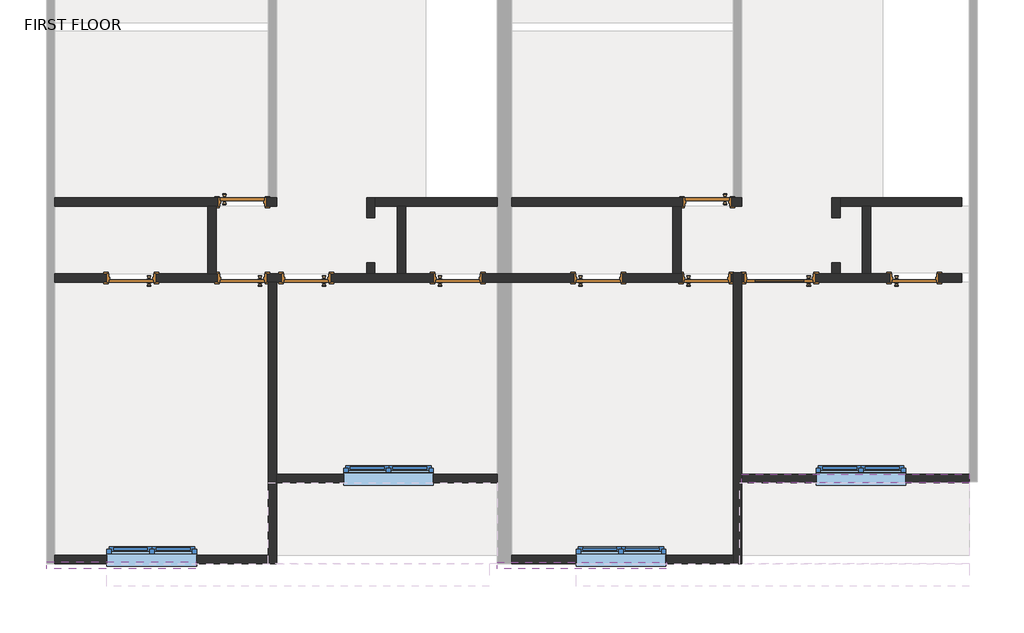
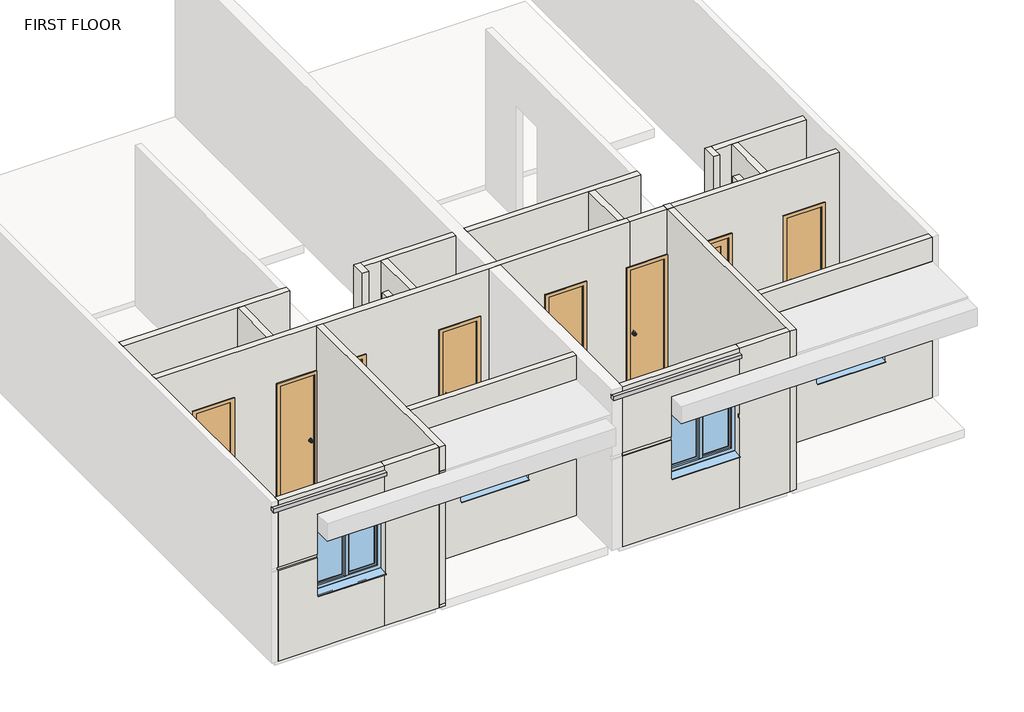
# One storey, part 1 of 2: 26 walls, 10 doors, 4 windows, 2 proxies.
"""IFC4 building model written with IfcOpenShell, lengths in millimetres."""

from ifc_helpers import new_model, si_unit, frame, origin, place, context, project, spatial, polyline, outline, extrude, faceted_brep, transform, mapped, element, save
from components import door_d4071c8b, door_c25f678d, door_03233f92, w2_0001_w2_2_f00e904a, w2_0001_w2_3_7b164e2c

model = new_model("IFC4")

# Units and contexts
model_context = context("Model", 3, world=origin())
ifc_project = project(units=[si_unit("LENGTHUNIT", "METRE", prefix="MILLI")], contexts=[model_context])

# Site, building, storey
site = spatial("IfcSite", under=ifc_project)
building = spatial("IfcBuilding", under=site)
storey = spatial("IfcBuildingStorey", under=building, Name="FIRST FLOOR", Elevation=3352.8)

# Proxies
placement = place(None, origin())
element("IfcBuildingElementProxy", 1, Name="Reveal 2", ObjectType="Reveal 2", at=placement, inside=storey, context=model_context, shape_type="SweptSolid", body=[
    extrude(outline(polyline([(-18263.2007021, -5496.2840801), (-18263.2007021, -5404.2090801), (-16237.550702, -5404.2090801), (-16237.550702, -5496.2840801), (-18263.2007021, -5496.2840801)])), frame((0.0, 0.0, 6248.4), z_axis=(0.0, 0.0, 1.0), x_axis=(1.0, 0.0, 0.0)), (0.0, 0.0, 1.0), 67.7333333),
])
element("IfcBuildingElementProxy", 2, Name="Reveal 2", ObjectType="Reveal 2", at=placement, inside=storey, context=model_context, shape_type="SweptSolid", body=[
    extrude(outline(polyline([(-9849.450702, -5405.2582515), (-9849.450702, -5497.3332515), (-12149.0934009, -5497.3332515), (-12149.0934009, -5405.2582515), (-9849.450702, -5405.2582515)])), frame((0.0, 0.0, 6248.4), z_axis=(0.0, 0.0, 1.0), x_axis=(1.0, 0.0, 0.0)), (0.0, 0.0, 1.0), 67.7333333),
])

# Doors
door_shape = door_d4071c8b(model_context)
element("IfcDoor", 3, ObjectType="Door-Interior-Single-2_Panel-Wood : 36\" x 84\"", at=placement, inside=storey, context=model_context, shape_type="MappedRepresentation", body=[
    mapped(door_shape, transform((-8312.7507021, -1552.9340801, 3352.8), x_axis=(-1.0, 0.0, 0.0), y_axis=(0.0, -1.0, 0.0), z_axis=(0.0, 0.0, 1.0))),
])
door_2_shape = door_c25f678d(model_context)
element("IfcDoor", 4, ObjectType="Door-Interior-Single-Flush_Panel-Wood : 24\" x 84\"", at=placement, inside=storey, context=model_context, shape_type="MappedRepresentation", body=[
    mapped(door_2_shape, transform((-17112.9480934, -1552.9340801, 3352.8), x_axis=(-1.0, 0.0, 0.0), y_axis=(0.0, -1.0, 0.0), z_axis=(0.0, 0.0, 1.0))),
])
element("IfcDoor", 5, ObjectType="Door-Interior-Single-Flush_Panel-Wood : 24\" x 84\"", at=placement, inside=storey, context=model_context, shape_type="MappedRepresentation", body=[
    mapped(door_2_shape, transform((-15607.9980934, -1552.9340801, 3352.8), x_axis=(-1.0, 0.0, 0.0), y_axis=(0.0, -1.0, 0.0), z_axis=(0.0, 0.0, 1.0))),
])
element("IfcDoor", 6, ObjectType="Door-Interior-Single-Flush_Panel-Wood : 24\" x 84\"", at=placement, inside=storey, context=model_context, shape_type="MappedRepresentation", body=[
    mapped(door_2_shape, transform((-14738.950702, -1552.9340801, 3352.8), x_axis=(-1.0, 0.0, 0.0), y_axis=(0.0, -1.0, 0.0), z_axis=(0.0, 0.0, 1.0))),
])
element("IfcDoor", 7, ObjectType="Door-Interior-Single-Flush_Panel-Wood : 24\" x 84\"", at=placement, inside=storey, context=model_context, shape_type="MappedRepresentation", body=[
    mapped(door_2_shape, transform((-15607.9980934, -517.8840801, 3352.8), x_axis=(1.0, 0.0, 0.0), y_axis=(0.0, 1.0, 0.0), z_axis=(0.0, 0.0, 1.0))),
])
door_3_shape = door_03233f92(model_context)
element("IfcDoor", 8, ObjectType="Door-Interior-Single-Flush_Panel-Wood : 24\" x 84\"", at=placement, inside=storey, context=model_context, shape_type="MappedRepresentation", body=[
    mapped(door_3_shape, transform((-9296.0980934, -517.8840801, 3352.8), x_axis=(-1.0, 0.0, 0.0), y_axis=(0.0, -1.0, 0.0), z_axis=(0.0, 0.0, 1.0))),
])
element("IfcDoor", 9, ObjectType="Door-Interior-Single-Flush_Panel-Wood : 24\" x 84\"", at=placement, inside=storey, context=model_context, shape_type="MappedRepresentation", body=[
    mapped(door_3_shape, transform((-9307.8954847, -1552.9340801, 3352.8), x_axis=(1.0, 0.0, 0.0), y_axis=(0.0, 1.0, 0.0), z_axis=(0.0, 0.0, 1.0))),
])
element("IfcDoor", 10, ObjectType="Door-Interior-Single-Flush_Panel-Wood : 24\" x 84\"", at=placement, inside=storey, context=model_context, shape_type="MappedRepresentation", body=[
    mapped(door_3_shape, transform((-10774.7454848, -1552.9340801, 3352.8), x_axis=(1.0, 0.0, 0.0), y_axis=(0.0, 1.0, 0.0), z_axis=(0.0, 0.0, 1.0))),
])
element("IfcDoor", 11, ObjectType="Door-Interior-Single-Flush_Panel-Wood : 24\" x 84\"", at=placement, inside=storey, context=model_context, shape_type="MappedRepresentation", body=[
    mapped(door_3_shape, transform((-6487.1257021, -1552.9340801, 3352.8), x_axis=(1.0, 0.0, 0.0), y_axis=(0.0, 1.0, 0.0), z_axis=(0.0, 0.0, 1.0))),
])
element("IfcDoor", 12, ObjectType="Door-Interior-Single-Flush_Panel-Wood : 24\" x 84\"", at=placement, inside=storey, context=model_context, shape_type="MappedRepresentation", body=[
    mapped(door_3_shape, transform((-12681.5507021, -1552.9340801, 3352.8), x_axis=(1.0, 0.0, 0.0), y_axis=(0.0, 1.0, 0.0), z_axis=(0.0, 0.0, 1.0))),
])

# Walls
element("IfcWall", 13, at=placement, inside=storey, context=model_context, shape_type="Brep", body=[
    faceted_brep([(-15139.0007021, -578.2090801, 6400.8), (-15962.6954847, -578.2090801, 6400.8), (-16076.9954847, -578.2090801, 6400.8), (-18148.9007021, -578.2090801, 6400.8), (-18148.9007021, -578.2090801, 3352.8), (-16076.9954847, -578.2090801, 3352.8), (-15962.6954847, -578.2090801, 3352.8), (-15938.1980934, -578.2090801, 3352.8), (-15938.1980934, -578.2090801, 5511.8), (-15277.7980934, -578.2090801, 5511.8), (-15277.7980934, -578.2090801, 3352.8), (-15139.0007021, -578.2090801, 3352.8), (-18148.9007021, -463.9090801, 6400.8), (-15253.3007021, -463.9090801, 6400.8), (-15139.0007021, -463.9090801, 6400.8), (-15139.0007021, -463.9090801, 3352.8), (-15253.3007021, -463.9090801, 3352.8), (-15277.7980934, -463.9090801, 3352.8), (-15277.7980934, -463.9090801, 5511.8), (-15938.1980934, -463.9090801, 5511.8), (-15938.1980934, -463.9090801, 3352.8), (-18148.9007021, -463.9090801, 3352.8)], [[[0, 1, 2, 3, 4, 5, 6, 7, 8, 9, 10, 11]], [[12, 13, 14, 15, 16, 17, 18, 19, 20, 21]], [[4, 21, 20, 7, 6, 5]], [[15, 11, 10, 17, 16]], [[3, 2, 1, 0, 14, 13, 12]], [[4, 3, 12, 21]], [[0, 11, 15, 14]], [[9, 18, 17, 10]], [[18, 9, 8, 19]], [[19, 8, 7, 20]]]),
])
element("IfcWall", 14, at=placement, inside=storey, context=model_context, shape_type="Brep", body=[
    faceted_brep([(-9612.6954847, -1606.9090801, 6400.8), (-11945.8934009, -1606.9090801, 6400.8), (-12149.0934009, -1606.9090801, 6400.8), (-15139.000702, -1606.9090801, 6400.8), (-15253.300702, -1606.9090801, 6400.8), (-18148.9007021, -1606.9090801, 6400.8), (-18148.9007021, -1606.9090801, 3352.8), (-17443.1480934, -1606.9090801, 3352.8), (-17443.1480934, -1606.9090801, 5511.8), (-16782.7480934, -1606.9090801, 5511.8), (-16782.7480934, -1606.9090801, 3352.8), (-15938.1980934, -1606.9090801, 3352.8), (-15938.1980934, -1606.9090801, 5511.8), (-15277.7980934, -1606.9090801, 5511.8), (-15277.7980934, -1606.9090801, 3352.8), (-15253.300702, -1606.9090801, 3352.8), (-15139.000702, -1606.9090801, 3352.8), (-15069.150702, -1606.9090801, 3352.8), (-15069.150702, -1606.9090801, 5511.8), (-14408.750702, -1606.9090801, 5511.8), (-14408.750702, -1606.9090801, 3352.8), (-13011.7507021, -1606.9090801, 3352.8), (-13011.7507021, -1606.9090801, 5511.8), (-12351.3507021, -1606.9090801, 5511.8), (-12351.3507021, -1606.9090801, 3352.8), (-12149.0934009, -1606.9090801, 3352.8), (-11945.8934009, -1606.9090801, 3352.8), (-11104.9454848, -1606.9090801, 3352.8), (-11104.9454848, -1606.9090801, 5511.8), (-10444.5454848, -1606.9090801, 5511.8), (-10444.5454848, -1606.9090801, 3352.8), (-9638.0954847, -1606.9090801, 3352.8), (-9638.0954847, -1606.9090801, 5511.8), (-9612.6954847, -1606.9090801, 5511.8), (-18148.9007021, -1492.6090801, 6400.8), (-16076.9954847, -1492.6090801, 6400.8), (-15962.6954847, -1492.6090801, 6400.8), (-13919.8007021, -1492.6090801, 6400.8), (-13805.5007021, -1492.6090801, 6400.8), (-13500.7007021, -1492.6090801, 6400.8), (-13386.4007021, -1492.6090801, 6400.8), (-12149.0934009, -1492.6090801, 6400.8), (-11945.8934009, -1492.6090801, 6400.8), (-9765.0954848, -1492.6090801, 6400.8), (-9650.7954848, -1492.6090801, 6400.8), (-9612.6954847, -1492.6090801, 6400.8), (-9612.6954847, -1492.6090801, 5511.8), (-9638.0954847, -1492.6090801, 5511.8), (-9638.0954847, -1492.6090801, 3352.8), (-9650.7954848, -1492.6090801, 3352.8), (-9765.0954848, -1492.6090801, 3352.8), (-10444.5454848, -1492.6090801, 3352.8), (-10444.5454848, -1492.6090801, 5511.8), (-11104.9454848, -1492.6090801, 5511.8), (-11104.9454848, -1492.6090801, 3352.8), (-11945.8934009, -1492.6090801, 3352.8), (-12149.0934009, -1492.6090801, 3352.8), (-12351.3507021, -1492.6090801, 3352.8), (-12351.3507021, -1492.6090801, 5511.8), (-13011.7507021, -1492.6090801, 5511.8), (-13011.7507021, -1492.6090801, 3352.8), (-13386.4007021, -1492.6090801, 3352.8), (-13500.7007021, -1492.6090801, 3352.8), (-13805.5007021, -1492.6090801, 3352.8), (-13919.8007021, -1492.6090801, 3352.8), (-14408.750702, -1492.6090801, 3352.8), (-14408.750702, -1492.6090801, 5511.8), (-15069.150702, -1492.6090801, 5511.8), (-15069.150702, -1492.6090801, 3352.8), (-15277.7980934, -1492.6090801, 3352.8), (-15277.7980934, -1492.6090801, 5511.8), (-15938.1980934, -1492.6090801, 5511.8), (-15938.1980934, -1492.6090801, 3352.8), (-15962.6954847, -1492.6090801, 3352.8), (-16076.9954847, -1492.6090801, 3352.8), (-16782.7480934, -1492.6090801, 3352.8), (-16782.7480934, -1492.6090801, 5511.8), (-17443.1480934, -1492.6090801, 5511.8), (-17443.1480934, -1492.6090801, 3352.8), (-18148.9007021, -1492.6090801, 3352.8)], [[[0, 1, 2, 3, 4, 5, 6, 7, 8, 9, 10, 11, 12, 13, 14, 15, 16, 17, 18, 19, 20, 21, 22, 23, 24, 25, 26, 27, 28, 29, 30, 31, 32, 33]], [[34, 35, 36, 37, 38, 39, 40, 41, 42, 43, 44, 45, 46, 47, 48, 49, 50, 51, 52, 53, 54, 55, 56, 57, 58, 59, 60, 61, 62, 63, 64, 65, 66, 67, 68, 69, 70, 71, 72, 73, 74, 75, 76, 77, 78, 79]], [[6, 79, 78, 7]], [[10, 75, 74, 73, 72, 11]], [[14, 69, 68, 17, 16, 15]], [[20, 65, 64, 63, 62, 61, 60, 21]], [[48, 31, 30, 51, 50, 49]], [[54, 27, 26, 25, 24, 57, 56, 55]], [[45, 0, 33, 46]], [[5, 4, 3, 2, 1, 0, 45, 44, 43, 42, 41, 40, 39, 38, 37, 36, 35, 34]], [[6, 5, 34, 79]], [[77, 8, 7, 78]], [[8, 77, 76, 9]], [[9, 76, 75, 10]], [[71, 12, 11, 72]], [[12, 71, 70, 13]], [[13, 70, 69, 14]], [[67, 18, 17, 68]], [[18, 67, 66, 19]], [[19, 66, 65, 20]], [[32, 47, 46, 33]], [[47, 32, 31, 48]], [[29, 52, 51, 30]], [[52, 29, 28, 53]], [[53, 28, 27, 54]], [[23, 58, 57, 24]], [[58, 23, 22, 59]], [[59, 22, 21, 60]]]),
])
element("IfcWall", 15, at=placement, inside=storey, context=model_context, shape_type="SweptSolid", body=[
    extrude(outline(polyline([(-16076.9954847, -1492.6090801), (-16076.9954847, -578.2090801), (-15962.6954847, -578.2090801), (-15962.6954847, -1492.6090801), (-16076.9954847, -1492.6090801)])), frame((0.0, 0.0, 3352.8), z_axis=(0.0, 0.0, 1.0), x_axis=(1.0, 0.0, 0.0)), (0.0, 0.0, 1.0), 3048.0),
])
element("IfcWall", 16, at=placement, inside=storey, context=model_context, shape_type="Brep", body=[
    faceted_brep([(-15139.000702, -5429.6090801, 3352.8), (-15139.000702, -4329.734083, 3352.8), (-15139.000702, -4215.434083, 3352.8), (-15139.000702, -1606.9090801, 3352.8), (-15139.000702, -1606.9090801, 3403.6), (-15139.000702, -5429.6090801, 3403.6), (-15253.300702, -5429.6090801, 3352.8), (-15253.300702, -5429.6090801, 3403.6), (-15253.300702, -1606.9090801, 3403.6), (-15253.300702, -1606.9090801, 3352.8), (-15253.300702, -5315.3090801, 3352.8)], [[[0, 1, 2, 3, 4, 5]], [[6, 7, 8, 9, 10]], [[3, 2, 1, 0, 6, 10, 9]], [[5, 4, 8, 7]], [[4, 3, 9, 8]], [[0, 5, 7, 6]]]),
])
element("IfcWall", 17, at=placement, inside=storey, context=model_context, shape_type="Brep", body=[
    faceted_brep([(-8827.100702, -5430.6582515, 3352.8), (-8827.100702, -4329.7340831, 3352.8), (-8827.100702, -4215.4340831, 3352.8), (-8827.100702, -1479.9090801, 3352.8), (-8827.100702, -1479.9090801, 6400.8), (-8827.100702, -4215.4340831, 6400.8), (-8827.100702, -4329.7340831, 6400.8), (-8827.100702, -5430.6582515, 6400.8), (-8941.400702, -5430.6582515, 3352.8), (-8941.400702, -5430.6582515, 6400.8), (-8941.400702, -5316.3582515, 6400.8), (-8941.400702, -1479.9090801, 6400.8), (-8941.400702, -1479.9090801, 3352.8), (-8941.400702, -5316.3582515, 3352.8)], [[[0, 1, 2, 3, 4, 5, 6, 7]], [[8, 9, 10, 11, 12, 13]], [[3, 2, 1, 0, 8, 13, 12]], [[4, 3, 12, 11]], [[7, 6, 5, 4, 11, 10, 9]], [[0, 7, 9, 8]]]),
])
element("IfcWall", 18, at=placement, inside=storey, context=model_context, shape_type="Brep", body=[
    faceted_brep([(-8827.1007021, -578.2090801, 6400.8), (-9650.7954848, -578.2090801, 6400.8), (-9765.0954848, -578.2090801, 6400.8), (-11945.8934009, -578.2090801, 6400.8), (-11945.8934009, -578.2090801, 3352.8), (-9765.0954848, -578.2090801, 3352.8), (-9650.7954848, -578.2090801, 3352.8), (-9626.2980934, -578.2090801, 3352.8), (-9626.2980934, -578.2090801, 5511.8), (-8965.8980934, -578.2090801, 5511.8), (-8965.8980934, -578.2090801, 3352.8), (-8827.1007021, -578.2090801, 3352.8), (-11945.8934009, -463.9090801, 6400.8), (-8941.4007021, -463.9090801, 6400.8), (-8827.1007021, -463.9090801, 6400.8), (-8827.1007021, -463.9090801, 3352.8), (-8941.4007021, -463.9090801, 3352.8), (-8965.8980934, -463.9090801, 3352.8), (-8965.8980934, -463.9090801, 5511.8), (-9626.2980934, -463.9090801, 5511.8), (-9626.2980934, -463.9090801, 3352.8), (-11945.8934009, -463.9090801, 3352.8)], [[[0, 1, 2, 3, 4, 5, 6, 7, 8, 9, 10, 11]], [[12, 13, 14, 15, 16, 17, 18, 19, 20, 21]], [[4, 21, 20, 7, 6, 5]], [[15, 11, 10, 17, 16]], [[3, 2, 1, 0, 14, 13, 12]], [[4, 3, 12, 21]], [[0, 11, 15, 14]], [[19, 8, 7, 20]], [[8, 19, 18, 9]], [[9, 18, 17, 10]]]),
])
element("IfcWall", 19, at=placement, inside=storey, context=model_context, shape_type="SweptSolid", body=[
    extrude(outline(polyline([(-9650.7954848, -578.2090801), (-9650.7954848, -1492.6090801), (-9765.0954848, -1492.6090801), (-9765.0954848, -578.2090801), (-9650.7954848, -578.2090801)])), frame((0.0, 0.0, 3352.8), z_axis=(0.0, 0.0, 1.0), x_axis=(1.0, 0.0, 0.0)), (0.0, 0.0, 1.0), 3048.0),
])
element("IfcWall", 20, at=placement, inside=storey, context=model_context, shape_type="Brep", body=[
    faceted_brep([(-9612.6954847, -1492.6090801, 6400.8), (-7607.9007021, -1492.6090801, 6400.8), (-7493.6007021, -1492.6090801, 6400.8), (-7188.8007021, -1492.6090801, 6400.8), (-7074.5007021, -1492.6090801, 6400.8), (-5842.6007021, -1492.6090801, 6400.8), (-5842.6007021, -1492.6090801, 3352.8), (-6156.9257021, -1492.6090801, 3352.8), (-6156.9257021, -1492.6090801, 5511.8), (-6817.3257021, -1492.6090801, 5511.8), (-6817.3257021, -1492.6090801, 3352.8), (-7074.5007021, -1492.6090801, 3352.8), (-7188.8007021, -1492.6090801, 3352.8), (-7493.6007021, -1492.6090801, 3352.8), (-7607.9007021, -1492.6090801, 3352.8), (-7830.1507021, -1492.6090801, 3352.8), (-7830.1507021, -1492.6090801, 5511.8), (-8795.3507021, -1492.6090801, 5511.8), (-8795.3507021, -1492.6090801, 3352.8), (-8977.6954847, -1492.6090801, 3352.8), (-8977.6954847, -1492.6090801, 5511.8), (-9612.6954847, -1492.6090801, 5511.8), (-5842.6007021, -1606.9090801, 6400.8), (-9612.6954847, -1606.9090801, 6400.8), (-9612.6954847, -1606.9090801, 5511.8), (-8977.6954847, -1606.9090801, 5511.8), (-8977.6954847, -1606.9090801, 3352.8), (-8795.3507021, -1606.9090801, 3352.8), (-8795.3507021, -1606.9090801, 5511.8), (-7830.1507021, -1606.9090801, 5511.8), (-7830.1507021, -1606.9090801, 3352.8), (-6817.3257021, -1606.9090801, 3352.8), (-6817.3257021, -1606.9090801, 5511.8), (-6156.9257021, -1606.9090801, 5511.8), (-6156.9257021, -1606.9090801, 3352.8), (-5842.6007021, -1606.9090801, 3352.8)], [[[0, 1, 2, 3, 4, 5, 6, 7, 8, 9, 10, 11, 12, 13, 14, 15, 16, 17, 18, 19, 20, 21]], [[22, 23, 24, 25, 26, 27, 28, 29, 30, 31, 32, 33, 34, 35]], [[6, 35, 34, 7]], [[26, 19, 18, 27]], [[10, 31, 30, 15, 14, 13, 12, 11]], [[23, 0, 21, 24]], [[5, 4, 3, 2, 1, 0, 23, 22]], [[6, 5, 22, 35]], [[25, 20, 19, 26]], [[20, 25, 24, 21]], [[33, 8, 7, 34]], [[8, 33, 32, 9]], [[9, 32, 31, 10]], [[17, 28, 27, 18]], [[28, 17, 16, 29]], [[29, 16, 15, 30]]]),
])
element("IfcWall", 21, at=placement, inside=storey, context=model_context, shape_type="Brep", body=[
    faceted_brep([(-7493.6007021, -730.6090801, 3352.8), (-7493.6007021, -578.2090801, 3352.8), (-7493.6007021, -463.9090801, 3352.8), (-7493.6007021, -463.9090801, 6400.8), (-7493.6007021, -578.2090801, 6400.8), (-7493.6007021, -730.6090801, 6400.8), (-7607.9007021, -730.6090801, 3352.8), (-7607.9007021, -730.6090801, 6400.8), (-7607.9007021, -463.9090801, 6400.8), (-7607.9007021, -463.9090801, 3352.8)], [[[0, 1, 2, 3, 4, 5]], [[6, 7, 8, 9]], [[2, 1, 0, 6, 9]], [[5, 4, 3, 8, 7]], [[0, 5, 7, 6]], [[3, 2, 9, 8]]]),
])
element("IfcWall", 22, at=placement, inside=storey, context=model_context, shape_type="Brep", body=[
    faceted_brep([(-7493.6007021, -578.2090801, 3352.8), (-7188.8007021, -578.2090801, 3352.8), (-7074.5007021, -578.2090801, 3352.8), (-5842.6007021, -578.2090801, 3352.8), (-5842.6007021, -578.2090801, 6400.8), (-7074.5007021, -578.2090801, 6400.8), (-7188.8007021, -578.2090801, 6400.8), (-7493.6007021, -578.2090801, 6400.8), (-7493.6007021, -463.9090801, 3352.8), (-7493.6007021, -463.9090801, 6400.8), (-5842.6007021, -463.9090801, 6400.8), (-5842.6007021, -463.9090801, 3352.8)], [[[0, 1, 2, 3, 4, 5, 6, 7]], [[8, 9, 10, 11]], [[3, 2, 1, 0, 8, 11]], [[4, 3, 11, 10]], [[7, 6, 5, 4, 10, 9]], [[0, 7, 9, 8]]]),
])
element("IfcWall", 23, at=placement, inside=storey, context=model_context, shape_type="SweptSolid", body=[
    extrude(outline(polyline([(-7493.6007021, -1340.2090801), (-7493.6007021, -1492.6090801), (-7607.9007021, -1492.6090801), (-7607.9007021, -1340.2090801), (-7493.6007021, -1340.2090801)])), frame((0.0, 0.0, 3352.8), z_axis=(0.0, 0.0, 1.0), x_axis=(1.0, 0.0, 0.0)), (0.0, 0.0, 1.0), 3048.0),
])
element("IfcWall", 24, at=placement, inside=storey, context=model_context, shape_type="SweptSolid", body=[
    extrude(outline(polyline([(-7074.5007021, -578.2090801), (-7074.5007021, -1492.6090801), (-7188.8007021, -1492.6090801), (-7188.8007021, -578.2090801), (-7074.5007021, -578.2090801)])), frame((0.0, 0.0, 3352.8), z_axis=(0.0, 0.0, 1.0), x_axis=(1.0, 0.0, 0.0)), (0.0, 0.0, 1.0), 3048.0),
])
element("IfcWall", 25, at=placement, inside=storey, context=model_context, shape_type="SweptSolid", body=[
    extrude(outline(polyline([(-13386.4007021, -578.2090801), (-13386.4007021, -1492.6090801), (-13500.7007021, -1492.6090801), (-13500.7007021, -578.2090801), (-13386.4007021, -578.2090801)])), frame((0.0, 0.0, 3352.8), z_axis=(0.0, 0.0, 1.0), x_axis=(1.0, 0.0, 0.0)), (0.0, 0.0, 1.0), 3048.0),
])
element("IfcWall", 26, at=placement, inside=storey, context=model_context, shape_type="Brep", body=[
    faceted_brep([(-13805.5007021, -730.6090801, 3352.8), (-13805.5007021, -578.2090801, 3352.8), (-13805.5007021, -463.9090801, 3352.8), (-13805.5007021, -463.9090801, 6400.8), (-13805.5007021, -578.2090801, 6400.8), (-13805.5007021, -730.6090801, 6400.8), (-13919.8007021, -730.6090801, 3352.8), (-13919.8007021, -730.6090801, 6400.8), (-13919.8007021, -463.9090801, 6400.8), (-13919.8007021, -463.9090801, 3352.8)], [[[0, 1, 2, 3, 4, 5]], [[6, 7, 8, 9]], [[2, 1, 0, 6, 9]], [[5, 4, 3, 8, 7]], [[0, 5, 7, 6]], [[3, 2, 9, 8]]]),
])
element("IfcWall", 27, at=placement, inside=storey, context=model_context, shape_type="Brep", body=[
    faceted_brep([(-13805.5007021, -578.2090801, 3352.8), (-13500.7007021, -578.2090801, 3352.8), (-13386.4007021, -578.2090801, 3352.8), (-12149.0934009, -578.2090801, 3352.8), (-12149.0934009, -578.2090801, 6400.8), (-13386.4007021, -578.2090801, 6400.8), (-13500.7007021, -578.2090801, 6400.8), (-13805.5007021, -578.2090801, 6400.8), (-13805.5007021, -463.9090801, 3352.8), (-13805.5007021, -463.9090801, 6400.8), (-12149.0934009, -463.9090801, 6400.8), (-12149.0934009, -463.9090801, 3352.8)], [[[0, 1, 2, 3, 4, 5, 6, 7]], [[8, 9, 10, 11]], [[3, 2, 1, 0, 8, 11]], [[7, 6, 5, 4, 10, 9]], [[0, 7, 9, 8]], [[4, 3, 11, 10]]]),
])
element("IfcWall", 28, at=placement, inside=storey, context=model_context, shape_type="SweptSolid", body=[
    extrude(outline(polyline([(-13805.5007021, -1340.2090801), (-13805.5007021, -1492.6090801), (-13919.8007021, -1492.6090801), (-13919.8007021, -1340.2090801), (-13805.5007021, -1340.2090801)])), frame((0.0, 0.0, 3352.8), z_axis=(0.0, 0.0, 1.0), x_axis=(1.0, 0.0, 0.0)), (0.0, 0.0, 1.0), 3048.0),
])
element("IfcWall", 29, at=placement, inside=storey, context=model_context, shape_type="SweptSolid", body=[
    extrude(outline(polyline([(3352.8, -15139.000702), (3352.8, -12149.0934009), (6400.8, -12149.0934009), (6400.8, -15139.000702), (3352.8, -15139.000702)]), holes=[polyline([(4352.8, -13012.2220515), (4352.8, -14231.4220515), (5612.8, -14231.4220515), (5612.8, -13012.2220515), (4352.8, -13012.2220515)])]), frame((0.0, -4329.734083, 0.0), z_axis=(0.0, 1.0, 0.0), x_axis=(0.0, 0.0, 1.0)), (0.0, 0.0, 1.0), 114.3),
])
element("IfcWall", 30, at=placement, inside=storey, context=model_context, shape_type="Brep", body=[
    faceted_brep([(-18148.9007021, -5429.6090801, 3352.8), (-16237.550702, -5429.6090801, 3352.8), (-16237.550702, -5429.6090801, 4352.8), (-17444.0507021, -5429.6090801, 4352.8), (-17444.0507021, -5429.6090801, 5072.38), (-18148.9007021, -5429.6090801, 5072.38), (-16237.550702, -5429.6090801, 6400.8), (-18148.9007021, -5429.6090801, 6400.8), (-18148.9007021, -5429.6090801, 6316.1333333), (-16237.550702, -5429.6090801, 6316.1333333), (-17444.0507021, -5429.6090801, 5572.0), (-16237.550702, -5429.6090801, 5572.0), (-16237.550702, -5429.6090801, 6248.4), (-18148.9007021, -5429.6090801, 6248.4), (-18148.9007021, -5429.6090801, 5140.1133333), (-17444.0507021, -5429.6090801, 5140.1133333), (-16237.550702, -5315.3090801, 3352.8), (-18148.9007021, -5315.3090801, 3352.8), (-18148.9007021, -5315.3090801, 6400.8), (-16237.550702, -5315.3090801, 6400.8), (-16237.550702, -5315.3090801, 5572.0), (-17444.0507021, -5315.3090801, 5572.0), (-17444.0507021, -5315.3090801, 4352.8), (-16237.550702, -5315.3090801, 4352.8), (-16237.550702, -5404.2090801, 6316.1333333), (-16237.550702, -5404.2090801, 6248.4), (-18148.9007021, -5404.2090801, 5072.38), (-18148.9007021, -5404.2090801, 5140.1133333), (-18148.9007021, -5404.2090801, 6248.4), (-18148.9007021, -5404.2090801, 6316.1333333), (-17444.0507021, -5404.2090801, 5140.1133333), (-17444.0507021, -5404.2090801, 5072.38)], [[[0, 1, 2, 3, 4, 5]], [[6, 7, 8, 9]], [[10, 11, 12, 13, 14, 15]], [[16, 17, 18, 19, 20, 21, 22, 23]], [[1, 0, 17, 16]], [[1, 16, 23, 2]], [[19, 6, 9, 24, 25, 12, 11, 20]], [[7, 6, 19, 18]], [[7, 18, 17, 0, 5, 26, 27, 14, 13, 28, 29, 8]], [[10, 21, 20, 11]], [[21, 10, 15, 30, 31, 4, 3, 22]], [[22, 3, 2, 23]], [[24, 9, 8, 29]], [[13, 12, 25, 28]], [[28, 25, 24, 29]], [[30, 27, 26, 31]], [[31, 26, 5, 4]], [[27, 30, 15, 14]]]),
])
element("IfcWall", 31, at=placement, inside=storey, context=model_context, shape_type="Brep", body=[
    faceted_brep([(-5742.8860997, -4215.4340831, 3352.8), (-8827.100702, -4215.4340831, 3352.8), (-8827.100702, -4215.4340831, 5638.8), (-5742.8860997, -4215.4340831, 5638.8), (-6600.1360997, -4215.4340831, 4352.8), (-6600.1360997, -4215.4340831, 5612.8), (-7819.3360997, -4215.4340831, 5612.8), (-7819.3360997, -4215.4340831, 4352.8), (-5742.8860997, -4329.7340831, 3352.8), (-5742.8860997, -4329.7340831, 5638.8), (-8827.100702, -4329.7340831, 5638.8), (-8827.100702, -4329.7340831, 3352.8), (-6600.1360997, -4329.7340831, 4352.8), (-7819.3360997, -4329.7340831, 4352.8), (-7819.3360997, -4329.7340831, 5612.8), (-6600.1360997, -4329.7340831, 5612.8), (-5742.8860997, -4318.3590801, 3352.8)], [[[0, 1, 2, 3], [4, 5, 6, 7]], [[8, 9, 10, 11], [12, 13, 14, 15]], [[1, 0, 16, 8, 11]], [[3, 2, 10, 9]], [[2, 1, 11, 10]], [[0, 3, 9, 8, 16]], [[5, 4, 12, 15]], [[6, 5, 15, 14]], [[7, 6, 14, 13]], [[4, 7, 13, 12]]]),
])
element("IfcWall", 32, at=placement, inside=storey, context=model_context, shape_type="Brep", body=[
    faceted_brep([(-8941.400702, -5316.3582515, 3352.8), (-9849.450702, -5316.3582515, 3352.8), (-9849.450702, -5316.3582515, 6400.8), (-8941.400702, -5316.3582515, 6400.8), (-8941.400702, -5430.6582515, 3352.8), (-8941.400702, -5430.6582515, 6400.8), (-9849.450702, -5430.6582515, 6400.8), (-9849.450702, -5430.6582515, 6316.1333333), (-9849.450702, -5430.6582515, 6248.4), (-9849.450702, -5430.6582515, 5140.1133333), (-9849.450702, -5430.6582515, 5072.38), (-9849.450702, -5430.6582515, 3352.8)], [[[0, 1, 2, 3]], [[4, 5, 6, 7, 8, 9, 10, 11]], [[1, 0, 4, 11]], [[2, 1, 11, 10, 9, 8, 7, 6]], [[3, 2, 6, 5]], [[0, 3, 5, 4]]]),
])
element("IfcWall", 33, at=placement, inside=storey, context=model_context, shape_type="Brep", body=[
    faceted_brep([(-15139.000702, -5429.6090801, 3403.6), (-15139.000702, -1606.9090801, 3403.6), (-15139.000702, -1606.9090801, 6400.8), (-15139.000702, -5429.6090801, 6400.8), (-15253.300702, -5429.6090801, 3403.6), (-15253.300702, -5429.6090801, 6400.8), (-15253.300702, -5315.3090801, 6400.8), (-15253.300702, -1606.9090801, 6400.8), (-15253.300702, -1606.9090801, 3403.6)], [[[0, 1, 2, 3]], [[4, 5, 6, 7, 8]], [[1, 0, 4, 8]], [[3, 2, 7, 6, 5]], [[0, 3, 5, 4]], [[2, 1, 8, 7]]]),
])
element("IfcWall", 34, at=placement, inside=storey, context=model_context, shape_type="Brep", body=[
    faceted_brep([(-16237.550702, -5429.6090801, 3352.8), (-15253.300702, -5429.6090801, 3352.8), (-15253.300702, -5429.6090801, 3403.6), (-15253.300702, -5429.6090801, 6400.8), (-16237.550702, -5429.6090801, 6400.8), (-16237.550702, -5429.6090801, 6316.1333333), (-16237.550702, -5429.6090801, 6248.4), (-16237.550702, -5429.6090801, 5572.0), (-16224.8507021, -5429.6090801, 5572.0), (-16224.8507021, -5429.6090801, 4352.8), (-16237.550702, -5429.6090801, 4352.8), (-15253.300702, -5315.3090801, 3352.8), (-16237.550702, -5315.3090801, 3352.8), (-16237.550702, -5315.3090801, 4352.8), (-16224.8507021, -5315.3090801, 4352.8), (-16224.8507021, -5315.3090801, 5572.0), (-16237.550702, -5315.3090801, 5572.0), (-16237.550702, -5315.3090801, 6400.8), (-15253.300702, -5315.3090801, 6400.8)], [[[0, 1, 2, 3, 4, 5, 6, 7, 8, 9, 10]], [[11, 12, 13, 14, 15, 16, 17, 18]], [[1, 0, 12, 11]], [[4, 3, 18, 17]], [[4, 17, 16, 7, 6, 5]], [[12, 0, 10, 13]], [[1, 11, 18, 3, 2]], [[14, 9, 8, 15]], [[15, 8, 7, 16]], [[9, 14, 13, 10]]]),
])
element("IfcWall", 35, at=placement, inside=storey, context=model_context, shape_type="Brep", body=[
    faceted_brep([(-9849.450702, -5316.3582515, 3352.8), (-11945.8934009, -5316.3582515, 3352.8), (-11945.8934009, -5316.3582515, 6400.8), (-9849.450702, -5316.3582515, 6400.8), (-11075.4720515, -5316.3582515, 4352.8), (-9856.2720515, -5316.3582515, 4352.8), (-9856.2720515, -5316.3582515, 5572.0), (-11075.4720515, -5316.3582515, 5572.0), (-11945.8934009, -5430.6582515, 3352.8), (-9849.450702, -5430.6582515, 3352.8), (-9849.450702, -5430.6582515, 5072.38), (-9856.2720515, -5430.6582515, 5072.38), (-9856.2720515, -5430.6582515, 4352.8), (-11075.4720515, -5430.6582515, 4352.8), (-11075.4720515, -5430.6582515, 5072.38), (-11945.8934009, -5430.6582515, 5072.38), (-9849.450702, -5430.6582515, 6400.8), (-11945.8934009, -5430.6582515, 6400.8), (-11945.8934009, -5430.6582515, 6316.1333333), (-9849.450702, -5430.6582515, 6316.1333333), (-11075.4720515, -5430.6582515, 5572.0), (-9856.2720515, -5430.6582515, 5572.0), (-9856.2720515, -5430.6582515, 5140.1133333), (-9849.450702, -5430.6582515, 5140.1133333), (-9849.450702, -5430.6582515, 6248.4), (-11945.8934009, -5430.6582515, 6248.4), (-11945.8934009, -5430.6582515, 5140.1133333), (-11075.4720515, -5430.6582515, 5140.1133333), (-9849.450702, -5405.2582515, 6316.1333333), (-9849.450702, -5405.2582515, 6248.4), (-9849.450702, -5405.2582515, 5140.1133333), (-9849.450702, -5405.2582515, 5072.38), (-11945.8934009, -5405.2582515, 5072.38), (-11945.8934009, -5405.2582515, 5140.1133333), (-11945.8934009, -5405.2582515, 6248.4), (-11945.8934009, -5405.2582515, 6316.1333333), (-11075.4720515, -5405.2582515, 5140.1133333), (-11075.4720515, -5405.2582515, 5072.38), (-9856.2720515, -5405.2582515, 5072.38), (-9856.2720515, -5405.2582515, 5140.1133333)], [[[0, 1, 2, 3], [4, 5, 6, 7]], [[8, 9, 10, 11, 12, 13, 14, 15]], [[16, 17, 18, 19]], [[20, 21, 22, 23, 24, 25, 26, 27]], [[1, 0, 9, 8]], [[3, 2, 17, 16]], [[0, 3, 16, 19, 28, 29, 24, 23, 30, 31, 10, 9]], [[2, 1, 8, 15, 32, 33, 26, 25, 34, 35, 18, 17]], [[5, 4, 13, 12]], [[4, 7, 20, 27, 36, 37, 14, 13]], [[7, 6, 21, 20]], [[6, 5, 12, 11, 38, 39, 22, 21]], [[35, 28, 19, 18]], [[29, 34, 25, 24]], [[28, 35, 34, 29]], [[39, 30, 23, 22]], [[31, 38, 11, 10]], [[30, 39, 38, 31]], [[33, 36, 27, 26]], [[37, 32, 15, 14]], [[36, 33, 32, 37]]]),
])
element("IfcWall", 36, at=placement, inside=storey, context=model_context, shape_type="SweptSolid", body=[
    extrude(outline(polyline([(-8827.100702, -4215.4340831), (-5742.8860997, -4215.4340831), (-5742.8860997, -4329.7340831), (-8827.100702, -4329.7340831), (-8827.100702, -4215.4340831)])), frame((0.0, 0.0, 5791.2), z_axis=(0.0, 0.0, 1.0), x_axis=(1.0, 0.0, 0.0)), (0.0, 0.0, 1.0), 152.4),
])
element("IfcWall", 37, at=placement, inside=storey, context=model_context, shape_type="Brep", body=[
    faceted_brep([(-5742.8860997, -4215.4340831, 5943.6), (-8827.100702, -4215.4340831, 5943.6), (-8827.100702, -4215.4340831, 6400.8), (-5742.8860997, -4215.4340831, 6400.8), (-5742.8860997, -4329.7340831, 5943.6), (-5742.8860997, -4329.7340831, 6400.8), (-8827.100702, -4329.7340831, 6400.8), (-8827.100702, -4329.7340831, 5943.6), (-5742.8860997, -4318.3590801, 6400.8)], [[[0, 1, 2, 3]], [[4, 5, 6, 7]], [[1, 0, 4, 7]], [[3, 2, 6, 5, 8]], [[0, 3, 8, 5, 4]], [[2, 1, 7, 6]]]),
])
element("IfcWall", 38, at=placement, inside=storey, context=model_context, shape_type="SweptSolid", body=[
    extrude(outline(polyline([(-8827.100702, -4215.4340831), (-5742.8860997, -4215.4340831), (-5742.8860997, -4329.7340831), (-8827.100702, -4329.7340831), (-8827.100702, -4215.4340831)])), frame((0.0, 0.0, 5638.8), z_axis=(0.0, 0.0, 1.0), x_axis=(1.0, 0.0, 0.0)), (0.0, 0.0, 1.0), 152.4),
])

# Windows
w2_0001_w2_2_shape = w2_0001_w2_2_f00e904a(model_context)
element("IfcWindow", 39, ObjectType="w2.0001 : w2 2", at=placement, inside=storey, context=model_context, shape_type="MappedRepresentation", body=[
    mapped(w2_0001_w2_2_shape, transform((-13621.8220515, -4272.584083, 3352.8), x_axis=(-1.0, 0.0, 0.0), y_axis=(0.0, -1.0, 0.0), z_axis=(0.0, 0.0, 1.0))),
])
element("IfcWindow", 40, ObjectType="w2.0001 : w2 2", at=placement, inside=storey, context=model_context, shape_type="MappedRepresentation", body=[
    mapped(w2_0001_w2_2_shape, transform((-7209.7360997, -4272.5840831, 3352.8), x_axis=(-1.0, 0.0, 0.0), y_axis=(0.0, -1.0, 0.0), z_axis=(0.0, 0.0, 1.0))),
])
w2_0001_w2_3_shape = w2_0001_w2_3_7b164e2c(model_context)
element("IfcWindow", 41, ObjectType="w2.0001 : w2 3", at=placement, inside=storey, context=model_context, shape_type="MappedRepresentation", body=[
    mapped(w2_0001_w2_3_shape, transform((-16834.4507021, -5372.4590801, 3352.8), x_axis=(-1.0, 0.0, 0.0), y_axis=(0.0, -1.0, 0.0), z_axis=(0.0, 0.0, 1.0))),
])
element("IfcWindow", 42, ObjectType="w2.0001 : w2 3", at=placement, inside=storey, context=model_context, shape_type="MappedRepresentation", body=[
    mapped(w2_0001_w2_3_shape, transform((-10465.8720515, -5373.5082515, 3352.8), x_axis=(-1.0, 0.0, 0.0), y_axis=(0.0, -1.0, 0.0), z_axis=(0.0, 0.0, 1.0))),
])

save(model, "model.ifc")

# Revit data of these elements
# Type "Door-Interior-Single-2_Panel-Wood : 36\" x 84\""
#   Type Mark = "9"
#   Assembly Code = "C1020300"
#   Analytic Construction = "Wooden"
#   Top Rail = 0' - 4 11/16"
#   Thickness = 0' - 1 3/8"
#   Thermal Resistance (R) = 2.5876 (h·ft²·°F)/BTU
#   Swing Angle [instance default] = 90.00°
#   Stiles = 0' - 4 3/4"
#   Rough Width = 3' - 2"
#   Rough Height = 7' - 1"
#   Lock Rail = 0' - 7 1/2"
#   Height = 7' - 0"
#   Width = 3' - 0"
#   Heat Transfer Coefficient (U) = 0.3865 BTU/(h·ft²·°F)
#   Bottom Rail = 0' - 9 1/8"
#   Trim Material = Cherry
#   Panel Material = Cherry
#   Frame Material = Cherry
#   Door Handle Material = Aluminum
#   Visual Light Transmittance = 0
#   Solar Heat Gain Coefficient = 0
#   Wall Closure = (empty or 0)
#   Function = (empty or 0)
# Type "Door-Interior-Single-Flush_Panel-Wood : 24\" x 84\""
#   Type Mark = "10"
#   Assembly Code = "C1020300"
#   Analytic Construction = "Wooden"
#   Thickness = 0' - 1 3/8"
#   Thermal Resistance (R) = 2.5876 (h·ft²·°F)/BTU
#   Swing Angle [instance default] = 90.00°
#   Rough Width = 2' - 2"
#   Rough Height = 7' - 1"
#   Height = 7' - 0"
#   Width = 2' - 0"
#   Heat Transfer Coefficient (U) = 0.3865 BTU/(h·ft²·°F)
#   Trim Material = Cherry
#   Panel Material = Cherry
#   Frame Material = Cherry
#   Door Handle Material = Aluminum
#   Visual Light Transmittance = 0
#   Solar Heat Gain Coefficient = 0
#   Wall Closure = (empty or 0)
#   Function = (empty or 0)
# Type
#   Assembly Code = "B2010"
# Type "w2.0001 : w2 2"
#   Type Mark = "20"
#   Operation = "DoublePanelVertical"
#   Keynote = "16.05.01"
#   Analytic Construction = "<None>"
#   Rough Width = 4' - 0"
#   Rough Height = 4' - 1.6063"
#   Rahmentiefe = 0' - 2.3622"
#   Rahmenhöhe unten = 0' - 3.14961"
#   Rahmehöhe oben = 0' - 3.14961"
#   Rahmenbreite = 0' - 2.3622"
#   Height = 4' - 1.6063"
#   Flügeltiefe = 0' - 2.3622"
#   Flügelbreite = 0' - 2.3622"
#   Einbautiefe (von außen) [instance default] = 0' - 5.51181"
#   Width = 4' - 0"
#   Kippflügel [instance default] = yes
#   Drehflügel im Grundriß darstellen [instance default] = no
#   Drehflügel [instance default] = yes
#   Define Thermal Properties by = 1
#   Rahmen [instance default] = none
#   Glas [instance default] = none
#   Flügel [instance default] = none
#   Fensterbank aussen [instance default] = none
#   Fensterbank innen [instance default] = none
#   Wall Closure = (empty or 0)
# Type "w2.0001 : w2 3"
#   Type Mark = "21"
#   Operation = "DoublePanelVertical"
#   Keynote = "16.05.01"
#   Analytic Construction = "<None>"
#   Rough Width = 4' - 0"
#   Rough Height = 4' - 0"
#   Rahmentiefe = 0' - 2.3622"
#   Rahmenhöhe unten = 0' - 3.14961"
#   Rahmehöhe oben = 0' - 3.14961"
#   Rahmenbreite = 0' - 2.3622"
#   Height = 4' - 0"
#   Flügeltiefe = 0' - 2.3622"
#   Flügelbreite = 0' - 2.3622"
#   Einbautiefe (von außen) [instance default] = 0' - 5.51181"
#   Width = 4' - 0"
#   Kippflügel [instance default] = yes
#   Drehflügel im Grundriß darstellen [instance default] = no
#   Drehflügel [instance default] = yes
#   Define Thermal Properties by = 1
#   Rahmen [instance default] = none
#   Glas [instance default] = none
#   Flügel [instance default] = none
#   Fensterbank aussen [instance default] = none
#   Fensterbank innen [instance default] = none
#   Wall Closure = (empty or 0)
# Element 3 (IfcDoor, "Door-Interior-Single-2_Panel-Wood : 36\" x 84\"")
#   Swing Angle = 90.00°
#   Phase Created = New Construction
#   Materials on its faces: "Cherry", "Aluminum"
# Elements 4, 5, 6, 7, 8, 9, 10, 11, 12 (IfcDoor, "Door-Interior-Single-Flush_Panel-Wood : 24\" x 84\"")
#   Swing Angle = 90.00°
#   Phase Created = New Construction
#   Materials on its faces: "Cherry", "Aluminum"
# Elements 13, 14, 15, 18, 19, 20, 21, 22, 23, 24, 25, 26, 27, 28, 35 (IfcWall)
#   Top Offset = 0' - 0"
#   Base Offset = 0' - 0"
#   wall height = 10' - 0"
#   Phase Created = New Construction
#   Base Constraint = FIRST FLOOR
#   Top Constraint = TOP OF ROOF
# Element 16 (IfcWall)
#   Top Offset = 0' - 0"
#   Base Offset = 0' - 0"
#   Unconnected Height = 0' - 2"
#   wall height = 0' - 2"
#   Phase Created = New Construction
#   Base Constraint = FIRST FLOOR
#   Materials on its faces: "red brown cladding"
# Elements 17, 29, 32, 34 (IfcWall)
#   Top Offset = 0' - 0"
#   Base Offset = 0' - 0"
#   wall height = 10' - 0"
#   Phase Created = New Construction
#   Base Constraint = FIRST FLOOR
#   Top Constraint = TOP OF ROOF
#   Materials on its faces: "red brown cladding"
# Element 30 (IfcWall)
#   Top Offset = 0' - 0"
#   Base Offset = 0' - 0"
#   wall height = 10' - 0"
#   Phase Created = New Construction
#   Base Constraint = FIRST FLOOR
#   Top Constraint = TOP OF ROOF
#   Materials on its faces: "Clad - White"
# Element 31 (IfcWall)
#   Top Offset = 0' - 0"
#   Base Offset = 0' - 0"
#   Unconnected Height = 7' - 6"
#   wall height = 7' - 6"
#   Phase Created = New Construction
#   Base Constraint = FIRST FLOOR
#   Materials on its faces: "red brown cladding"
# Element 33 (IfcWall)
#   built-in parameter 1001111 = 0' - 2"
#   Top Offset = 0' - 0"
#   Base Offset = 0' - 2"
#   Unconnected Height = 9' - 10"
#   wall height = 9' - 10"
#   Phase Created = New Construction
#   Base Constraint = FIRST FLOOR
#   Top Constraint = TOP OF ROOF
#   Materials on its faces: "red brown cladding"
# Element 36 (IfcWall)
#   built-in parameter 1001111 = 8' - 0"
#   Top Offset = 0' - 0"
#   Base Offset = 8' - 0"
#   Unconnected Height = 0' - 6"
#   wall height = 0' - 6"
#   Phase Created = New Construction
#   Base Constraint = FIRST FLOOR
#   Materials on its faces: "red brown cladding"
# Element 37 (IfcWall)
#   built-in parameter 1001111 = 8' - 6"
#   Top Offset = 0' - 0"
#   Base Offset = 8' - 6"
#   Unconnected Height = 1' - 6"
#   wall height = 1' - 6"
#   Phase Created = New Construction
#   Base Constraint = FIRST FLOOR
#   Top Constraint = TOP OF ROOF
#   Materials on its faces: "red brown cladding"
# Element 38 (IfcWall)
#   built-in parameter 1001111 = 7' - 6"
#   Top Offset = 0' - 0"
#   Base Offset = 7' - 6"
#   Unconnected Height = 0' - 6"
#   wall height = 0' - 6"
#   Phase Created = New Construction
#   Base Constraint = FIRST FLOOR
#   Materials on its faces: "red brown cladding"
# Element 39 (IfcWindow, "w2.0001 : w2 2")
#   Mark = "10"
#   Einbautiefe (von außen) = 0' - 5.51181"
#   Kippflügel = yes
#   Drehflügel im Grundriß darstellen = no
#   Drehflügel = yes
#   Rahmen = none
#   Glas = none
#   Flügel = none
#   Fensterbank innen = none
#   Fensterbank aussen = none
#   Phase Created = New Construction
#   Materials on its faces: "Fenster - Kunststoff", "Fenster - Kunststoff weiss", "Glass", "Fenster - Holz"
# Element 40 (IfcWindow, "w2.0001 : w2 2")
#   Mark = "11"
#   Einbautiefe (von außen) = 0' - 5.51181"
#   Kippflügel = yes
#   Drehflügel im Grundriß darstellen = no
#   Drehflügel = yes
#   Rahmen = none
#   Glas = none
#   Flügel = none
#   Fensterbank innen = none
#   Fensterbank aussen = none
#   Phase Created = New Construction
#   Materials on its faces: "Fenster - Kunststoff", "Fenster - Kunststoff weiss", "Glass", "Fenster - Holz"
# Element 41 (IfcWindow, "w2.0001 : w2 3")
#   Mark = "8"
#   Einbautiefe (von außen) = 0' - 5.51181"
#   Kippflügel = yes
#   Drehflügel im Grundriß darstellen = no
#   Drehflügel = yes
#   Rahmen = none
#   Glas = none
#   Flügel = none
#   Fensterbank innen = none
#   Fensterbank aussen = none
#   Phase Created = New Construction
#   Materials on its faces: "Fenster - Kunststoff", "Fenster - Kunststoff weiss", "Glass", "Fenster - Holz"
# Element 42 (IfcWindow, "w2.0001 : w2 3")
#   Mark = "9"
#   Einbautiefe (von außen) = 0' - 5.51181"
#   Kippflügel = yes
#   Drehflügel im Grundriß darstellen = no
#   Drehflügel = yes
#   Rahmen = none
#   Glas = none
#   Flügel = none
#   Fensterbank innen = none
#   Fensterbank aussen = none
#   Phase Created = New Construction
#   Materials on its faces: "Fenster - Kunststoff", "Fenster - Kunststoff weiss", "Glass", "Fenster - Holz"
# Materials
#   "Cherry": class "Wood", colour RGB 226 177 128, transparency 0, Description = "Prunus Serotina", Cost = 0
#   "Aluminum": class "Metal", colour RGB 247 247 247, transparency 0, Description = "Aluminum 6061", Cost = 0
#   "red brown cladding": class "Generic", colour RGB 151 67 57, transparency 0, Cost = 0
#   "Clad - White": class "Wood", colour RGB 242 242 238, transparency 0, Cost = 0
#   "Fenster - Kunststoff": colour RGB 249 249 249, transparency 0
#   "Fenster - Kunststoff weiss": colour RGB 249 249 249, transparency 0
#   "Glass": class "Glass", colour RGB 0 128 192, transparency 0.75, Description = "Soda Lime Glass", Cost = 0
#   "Fenster - Holz": colour RGB 216 135 75, transparency 0
